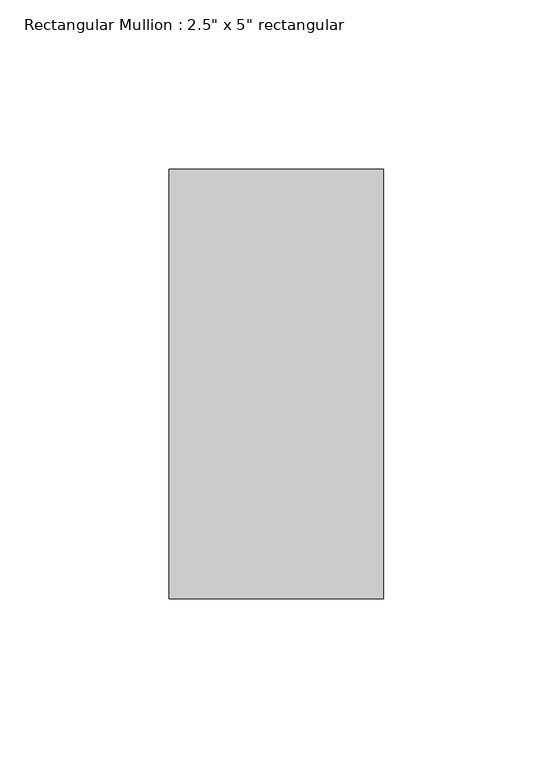
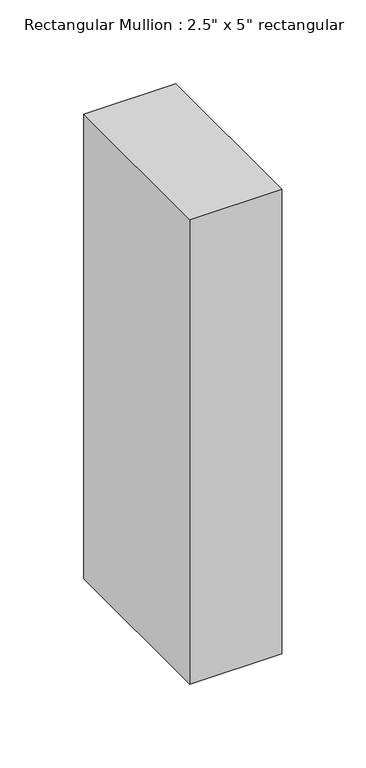
"""IFC4 building model written with IfcOpenShell, lengths in millimetres: member geometry."""

from ifc_helpers import new_model, si_unit, frame, origin, place, context, project, spatial, polyline, outline, extrude, source, transform, mapped, element, save


def member_c2e216af(model_context):
    return source(origin(), model_context, "Body", "SweptSolid", [
        extrude(outline(polyline([(31.75, 63.5), (31.75, -63.5), (-31.75, -63.5), (-31.75, 63.5), (31.75, 63.5)])), frame((0.0, 0.0, -338.9748327), z_axis=(0.0, 0.0, 1.0), x_axis=(1.0, 0.0, 0.0)), (0.0, 0.0, 1.0), 338.9748327),
    ])


if __name__ == "__main__":
    model = new_model("IFC4")
    model_context = context("Model", 3, world=origin())
    ifc_project = project(units=[si_unit("LENGTHUNIT", "METRE", prefix="MILLI")], contexts=[model_context])
    site = spatial("IfcSite", under=ifc_project)
    building = spatial("IfcBuilding", under=site)
    placement = place(None, origin())
    member_shape = member_c2e216af(model_context)
    element("IfcMember", 1, ObjectType="Rectangular Mullion : 2.5\" x 5\" rectangular", at=placement, inside=building, context=model_context, shape_type="MappedRepresentation", body=[
        mapped(member_shape, transform((0.0, 0.0, 0.0), x_axis=(1.0, 0.0, 0.0), y_axis=(0.0, 1.0, 0.0), z_axis=(0.0, 0.0, 1.0))),
    ])
    save(model, "model.ifc")

# Revit data of these elements
# Type "Rectangular Mullion : 2.5\" x 5\" rectangular"
#   built-in parameter 1007304 = 0.416667 (stored number, unit not read)
#   built-in parameter 1007301 = 0.104167 (stored number, unit not read)
#   built-in parameter 1007300 = 0.104167 (stored number, unit not read)
# Element 1 (IfcMember, "Rectangular Mullion : 2.5\" x 5\" rectangular")
#   Materials on its faces: "Aluminum"
# Materials
#   "Aluminum": class "Metal", colour RGB 247 247 247, transparency 0, Description = "Aluminum 6061", Cost = 0
